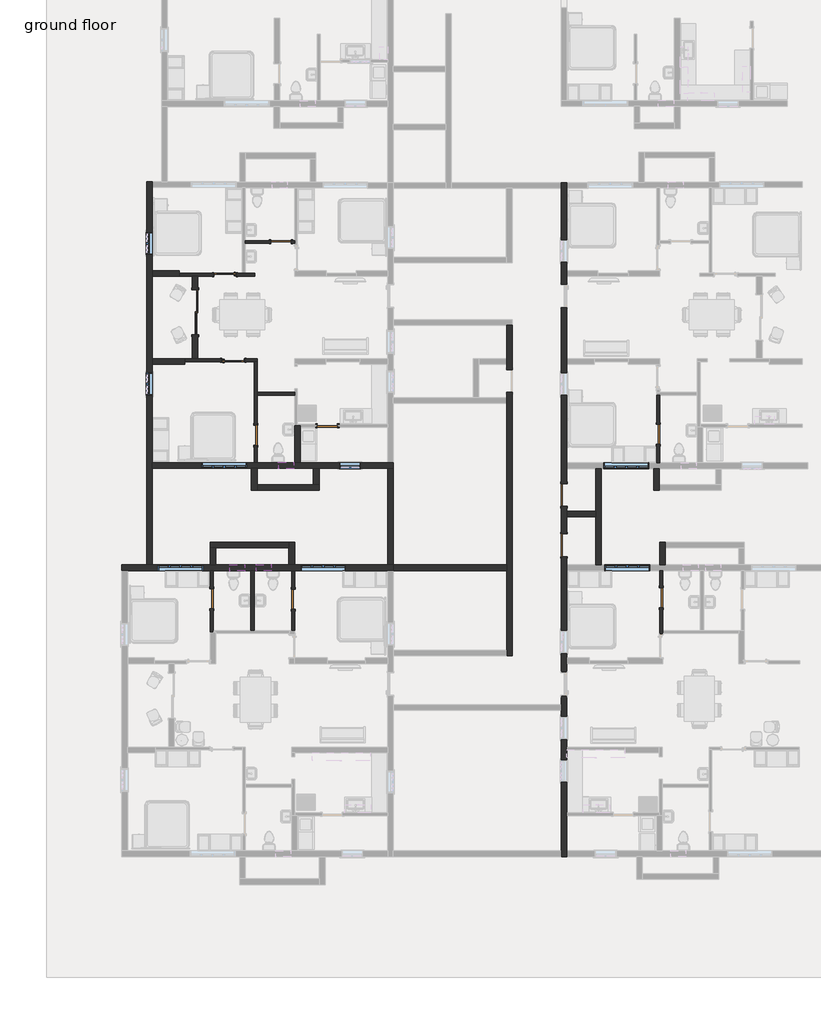
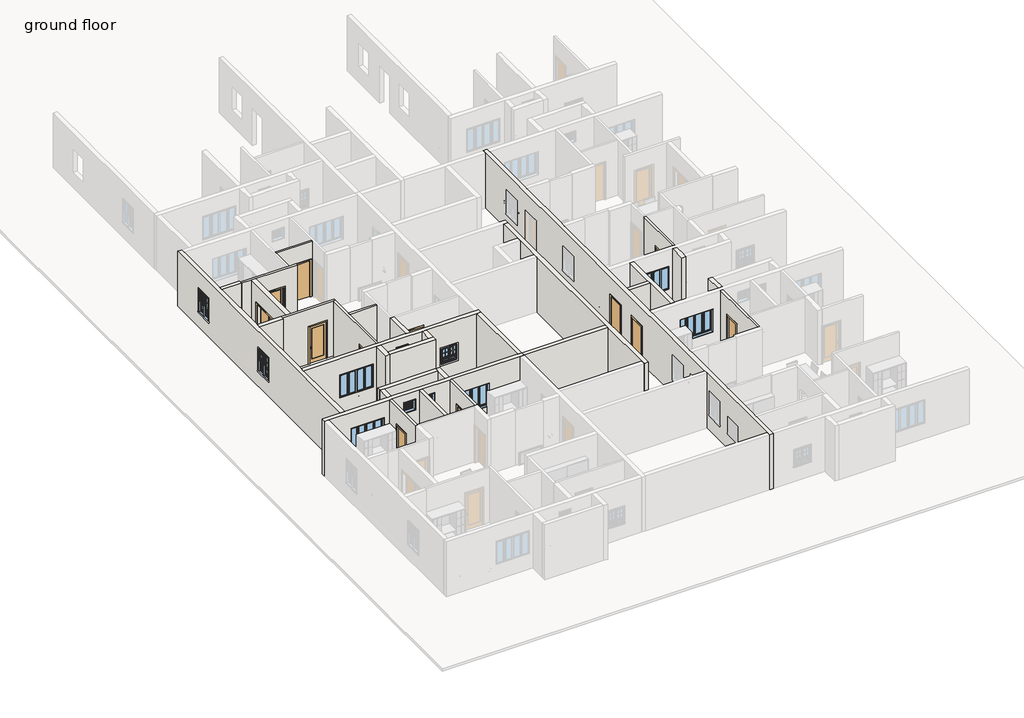
# One storey, part 2 of 16: 31 walls, 12 doors, 11 windows.
"""IFC4 building model written with IfcOpenShell, lengths in millimetres."""

from ifc_helpers import new_model, si_unit, frame, origin, place, context, project, spatial, polyline, outline, extrude, faceted_brep, transform, mapped, element, save
from components import door_d4d75d1e, door_a3feeac7, door_38851409, door_d141acb4, door_0ca8825f, window_ced37e8f, window_5487fb6d, window_f2d8fef0, window_45970670

model = new_model("IFC4")

# Units and contexts
model_context = context("Model", 3, world=origin())
ifc_project = project(units=[si_unit("LENGTHUNIT", "METRE", prefix="MILLI")], contexts=[model_context])

# Site, building, storey
site = spatial("IfcSite", under=ifc_project)
building = spatial("IfcBuilding", under=site)
storey = spatial("IfcBuildingStorey", under=building, Name="ground floor", Elevation=609.6)

# Doors
placement = place(None, origin())
door_shape = door_d4d75d1e(model_context)
element("IfcDoor", 1, ObjectType="Door-Double-Sliding : 72\" x 84\"", at=placement, inside=storey, context=model_context, shape_type="MappedRepresentation", body=[
    mapped(door_shape, transform((44373.526243, -3261.4613664, 609.6), x_axis=(0.0, -1.0, 0.0), y_axis=(1.0, 0.0, 0.0), z_axis=(0.0, 0.0, 1.0))),
])
door_2_shape = door_a3feeac7(model_context)
element("IfcDoor", 2, ObjectType="Door-Interior-Single-1_Panel-Wood : 36\" x 84\"", at=placement, inside=storey, context=model_context, shape_type="MappedRepresentation", body=[
    mapped(door_2_shape, transform((45713.376243, -1734.2863664, 609.6), x_axis=(-1.0, 0.0, 0.0), y_axis=(0.0, -1.0, 0.0), z_axis=(0.0, 0.0, 1.0))),
])
element("IfcDoor", 3, ObjectType="Door-Interior-Single-1_Panel-Wood : 36\" x 84\"", at=placement, inside=storey, context=model_context, shape_type="MappedRepresentation", body=[
    mapped(door_2_shape, transform((46043.576243, -5207.7363664, 609.6), x_axis=(1.0, 0.0, 0.0), y_axis=(0.0, 1.0, 0.0), z_axis=(0.0, 0.0, 1.0))),
])
door_3_shape = door_38851409(model_context)
element("IfcDoor", 4, ObjectType="Single-Flush : 32\" x 84\"", at=placement, inside=storey, context=model_context, shape_type="MappedRepresentation", body=[
    mapped(door_3_shape, transform((63299.8812819, -8216.4424723, 609.6), x_axis=(0.0, 1.0, 0.0), y_axis=(-1.0, 0.0, 0.0), z_axis=(0.0, 0.0, 1.0))),
])
element("IfcDoor", 5, ObjectType="Single-Flush : 32\" x 84\"", at=placement, inside=storey, context=model_context, shape_type="MappedRepresentation", body=[
    mapped(door_3_shape, transform((46957.976243, -8252.8253443, 609.6), x_axis=(0.0, 1.0, 0.0), y_axis=(-1.0, 0.0, 0.0), z_axis=(0.0, 0.0, 1.0))),
])
element("IfcDoor", 6, ObjectType="Single-Flush : 32\" x 84\"", at=placement, inside=storey, context=model_context, shape_type="MappedRepresentation", body=[
    mapped(door_3_shape, transform((47986.676243, -403.9613664, 609.6), x_axis=(-1.0, 0.0, 0.0), y_axis=(0.0, -1.0, 0.0), z_axis=(0.0, 0.0, 1.0))),
])
element("IfcDoor", 7, ObjectType="Single-Flush : 32\" x 84\"", at=placement, inside=storey, context=model_context, shape_type="MappedRepresentation", body=[
    mapped(door_3_shape, transform((48486.1657505, -14903.6865909, 609.6), x_axis=(0.0, -1.0, 0.0), y_axis=(1.0, 0.0, 0.0), z_axis=(0.0, 0.0, 1.0))),
])
door_4_shape = door_d141acb4(model_context)
element("IfcDoor", 8, ObjectType="Single-Flush : 32\" x 84\"", at=placement, inside=storey, context=model_context, shape_type="MappedRepresentation", body=[
    mapped(door_4_shape, transform((49872.626243, -7858.8613664, 609.6), x_axis=(-1.0, 0.0, 0.0), y_axis=(0.0, -1.0, 0.0), z_axis=(0.0, 0.0, 1.0))),
])
element("IfcDoor", 9, ObjectType="Single-Flush : 32\" x 84\"", at=placement, inside=storey, context=model_context, shape_type="MappedRepresentation", body=[
    mapped(door_4_shape, transform((63414.1812819, -14846.5365909, 609.6), x_axis=(0.0, -1.0, 0.0), y_axis=(1.0, 0.0, 0.0), z_axis=(0.0, 0.0, 1.0))),
])
element("IfcDoor", 10, ObjectType="Single-Flush : 32\" x 84\"", at=placement, inside=storey, context=model_context, shape_type="MappedRepresentation", body=[
    mapped(door_4_shape, transform((45170.5764835, -14881.4615909, 609.6), x_axis=(0.0, -1.0, 0.0), y_axis=(1.0, 0.0, 0.0), z_axis=(0.0, 0.0, 1.0))),
])
door_5_shape = door_0ca8825f(model_context)
element("IfcDoor", 11, ObjectType="Single-Flush : 36\" x 84\"", at=placement, inside=storey, context=model_context, shape_type="MappedRepresentation", body=[
    mapped(door_5_shape, transform((59470.8312819, -10676.4239787, 609.6), x_axis=(0.0, 1.0, 0.0), y_axis=(-1.0, 0.0, 0.0), z_axis=(0.0, 0.0, 1.0))),
])
element("IfcDoor", 12, ObjectType="Single-Flush : 36\" x 84\"", at=placement, inside=storey, context=model_context, shape_type="MappedRepresentation", body=[
    mapped(door_5_shape, transform((59470.8312819, -12712.9365909, 609.6), x_axis=(0.0, 1.0, 0.0), y_axis=(-1.0, 0.0, 0.0), z_axis=(0.0, 0.0, 1.0))),
])

# Walls
element("IfcWall", 13, ObjectType="Generic - 4.5\"", at=placement, inside=storey, context=model_context, shape_type="Brep", body=[
    faceted_brep([(43851.5274525, -1680.3113664, 609.6), (43851.5274525, -1680.3113664, 3810.0), (46418.226243, -1680.3113664, 3810.0), (46532.526243, -1680.3113664, 3810.0), (46913.6306279, -1680.3113664, 3810.0), (46913.6306279, -1680.3113664, 609.6), (46532.526243, -1680.3113664, 609.6), (46418.226243, -1680.3113664, 609.6), (46195.976243, -1680.3113664, 609.6), (46195.976243, -1680.3113664, 2768.6), (45230.776243, -1680.3113664, 2768.6), (45230.776243, -1680.3113664, 609.6), (43851.5274525, -1794.6113664, 3810.0), (43851.5274525, -1794.6113664, 609.6), (44386.226243, -1794.6113664, 609.6), (44614.826243, -1794.6113664, 609.6), (45230.776243, -1794.6113664, 609.6), (45230.776243, -1794.6113664, 2768.6), (46195.976243, -1794.6113664, 2768.6), (46195.976243, -1794.6113664, 609.6), (46913.6306279, -1794.6113664, 609.6), (46913.6306279, -1794.6113664, 3810.0), (44614.826243, -1794.6113664, 3810.0), (44386.226243, -1794.6113664, 3810.0)], [[[0, 1, 2, 3, 4, 5, 6, 7, 8, 9, 10, 11]], [[12, 13, 14, 15, 16, 17, 18, 19, 20, 21, 22, 23]], [[5, 20, 19, 8, 7, 6]], [[13, 0, 11, 16, 15, 14]], [[1, 0, 13, 12]], [[4, 3, 2, 1, 12, 23, 22, 21]], [[5, 4, 21, 20]], [[10, 17, 16, 11]], [[17, 10, 9, 18]], [[18, 9, 8, 19]]]),
])
element("IfcWall", 14, ObjectType="Generic - 4.5\"", at=placement, inside=storey, context=model_context, shape_type="SweptSolid", body=[
    extrude(outline(polyline([(609.6, 46532.526243), (609.6, 47580.276243), (2743.2, 47580.276243), (2743.2, 48393.076243), (609.6, 48393.076243), (609.6, 48539.126243), (3810.0, 48539.126243), (3810.0, 46532.526243), (609.6, 46532.526243)])), frame((0.0, -461.1113664, 0.0), z_axis=(0.0, 1.0, 0.0), x_axis=(0.0, 0.0, 1.0)), (0.0, 0.0, 1.0), 114.3),
])
element("IfcWall", 15, ObjectType="Generic - 4.5\"", at=placement, inside=storey, context=model_context, shape_type="Brep", body=[
    faceted_brep([(47015.126243, -5261.7113664, 3810.0), (46900.826243, -5261.7113664, 3810.0), (44081.426243, -5261.7113664, 3810.0), (44081.426243, -5261.7113664, 609.6), (45560.976243, -5261.7113664, 609.6), (45560.976243, -5261.7113664, 2768.6), (46526.176243, -5261.7113664, 2768.6), (46526.176243, -5261.7113664, 609.6), (46900.826243, -5261.7113664, 609.6), (47015.126243, -5261.7113664, 609.6), (44081.426243, -5147.4113664, 3810.0), (44386.226243, -5147.4113664, 3810.0), (44614.826243, -5147.4113664, 3810.0), (47015.126243, -5147.4113664, 3810.0), (47015.126243, -5147.4113664, 609.6), (46526.176243, -5147.4113664, 609.6), (46526.176243, -5147.4113664, 2768.6), (45560.976243, -5147.4113664, 2768.6), (45560.976243, -5147.4113664, 609.6), (44614.826243, -5147.4113664, 609.6), (44386.226243, -5147.4113664, 609.6), (44081.426243, -5147.4113664, 609.6)], [[[0, 1, 2, 3, 4, 5, 6, 7, 8, 9]], [[10, 11, 12, 13, 14, 15, 16, 17, 18, 19, 20, 21]], [[3, 21, 20, 19, 18, 4]], [[14, 9, 8, 7, 15]], [[2, 1, 0, 13, 12, 11, 10]], [[3, 2, 10, 21]], [[0, 9, 14, 13]], [[6, 16, 15, 7]], [[16, 6, 5, 17]], [[17, 5, 4, 18]]]),
])
element("IfcWall", 16, ObjectType="Generic - 4.5\"", at=placement, inside=storey, context=model_context, shape_type="Brep", body=[
    faceted_brep([(46900.826243, -5261.7113664, 609.6), (46900.826243, -7846.4253443, 609.6), (46900.826243, -7846.4253443, 2743.2), (46900.826243, -8659.2253443, 2743.2), (46900.826243, -8659.2253443, 609.6), (46900.826243, -9357.7253443, 609.6), (46900.826243, -9357.7253443, 3810.0), (46900.826243, -5261.7113664, 3810.0), (47015.126243, -7846.4253443, 2743.2), (47015.126243, -7846.4253443, 609.6), (47015.126243, -6620.6113664, 609.6), (47015.126243, -6506.3113664, 609.6), (47015.126243, -5261.7113664, 609.6), (47015.126243, -5261.7113664, 3810.0), (47015.126243, -6506.3113664, 3810.0), (47015.126243, -6620.6113664, 3810.0), (47015.126243, -9357.7253443, 3810.0), (47015.126243, -9357.7253443, 609.6), (47015.126243, -8659.2253443, 609.6), (47015.126243, -8659.2253443, 2743.2)], [[[0, 1, 2, 3, 4, 5, 6, 7]], [[8, 9, 10, 11, 12, 13, 14, 15, 16, 17, 18, 19]], [[18, 17, 5, 4]], [[12, 11, 10, 9, 1, 0]], [[7, 6, 16, 15, 14, 13]], [[0, 7, 13, 12]], [[6, 5, 17, 16]], [[2, 1, 9, 8]], [[3, 2, 8, 19]], [[4, 3, 19, 18]]]),
])
element("IfcWall", 17, ObjectType="Generic - 4.5\"", at=placement, inside=storey, context=model_context, shape_type="SweptSolid", body=[
    extrude(outline(polyline([(48539.126243, -6620.6113664), (47015.126243, -6620.6113664), (47015.126243, -6506.3113664), (48539.126243, -6506.3113664), (48539.126243, -6620.6113664)])), frame((0.0, 0.0, 609.6), z_axis=(0.0, 0.0, 1.0), x_axis=(1.0, 0.0, 0.0)), (0.0, 0.0, 1.0), 3200.4),
])
element("IfcWall", 18, ObjectType="Generic - 4.5\"", at=placement, inside=storey, context=model_context, shape_type="SweptSolid", body=[
    extrude(outline(polyline([(-6620.6113664, 609.6), (-7810.0424723, 609.6), (-7810.0424723, 2743.2), (-8622.8424723, 2743.2), (-8622.8424723, 609.6), (-9372.1424723, 609.6), (-9372.1424723, 3810.0), (-6620.6113664, 3810.0), (-6620.6113664, 609.6)])), frame((63242.7312819, 0.0, 0.0), z_axis=(1.0, 0.0, 0.0), x_axis=(0.0, 1.0, 0.0)), (0.0, 0.0, 1.0), 114.3),
])
element("IfcWall", 19, ObjectType="Generic - 4.5\"", at=placement, inside=storey, context=model_context, shape_type="Brep", body=[
    faceted_brep([(45113.4264835, -15287.8615909, 2743.2), (45113.4264835, -15287.8615909, 609.6), (45113.4264835, -16237.1865909, 609.6), (45113.4264835, -16237.1865909, 3810.0), (45113.4264835, -13741.6365909, 3810.0), (45113.4264835, -13741.6365909, 609.6), (45113.4264835, -14475.0615909, 609.6), (45113.4264835, -14475.0615909, 2743.2), (45227.7264835, -16237.1865909, 609.6), (45227.7264835, -16180.0365909, 609.6), (45227.7264835, -15287.8615909, 609.6), (45227.7264835, -15287.8615909, 2743.2), (45227.7264835, -14475.0615909, 2743.2), (45227.7264835, -14475.0615909, 609.6), (45227.7264835, -13741.6365909, 609.6), (45227.7264835, -13741.6365909, 3810.0), (45227.7264835, -16180.0365909, 3810.0), (45227.7264835, -16237.1865909, 3810.0)], [[[0, 1, 2, 3, 4, 5, 6, 7]], [[8, 9, 10, 11, 12, 13, 14, 15, 16, 17]], [[6, 5, 14, 13]], [[2, 1, 10, 9, 8]], [[3, 2, 8, 17]], [[4, 3, 17, 16, 15]], [[5, 4, 15, 14]], [[11, 10, 1, 0]], [[12, 11, 0, 7]], [[13, 12, 7, 6]]]),
])
element("IfcWall", 20, ObjectType="Generic - 4.5\"", at=placement, inside=storey, context=model_context, shape_type="SweptSolid", body=[
    extrude(outline(polyline([(-15310.0865909, 2743.2), (-15310.0865909, 609.6), (-16180.0365909, 609.6), (-16180.0365909, 3810.0), (-13741.6365909, 3810.0), (-13741.6365909, 609.6), (-14497.2865909, 609.6), (-14497.2865909, 2743.2), (-15310.0865909, 2743.2)])), frame((48429.0157505, 0.0, 0.0), z_axis=(1.0, 0.0, 0.0), x_axis=(0.0, 1.0, 0.0)), (0.0, 0.0, 1.0), 114.3),
])
element("IfcWall", 21, ObjectType="Generic - 4.5\"", at=placement, inside=storey, context=model_context, shape_type="Brep", body=[
    faceted_brep([(63357.0312819, -15252.9365909, 2743.2), (63357.0312819, -15252.9365909, 609.6), (63357.0312819, -16335.6115909, 609.6), (63357.0312819, -16335.6115909, 2768.6), (63357.0312819, -17284.9365909, 2768.6), (63357.0312819, -17284.9365909, 3810.0), (63357.0312819, -13741.6365909, 3810.0), (63357.0312819, -13741.6365909, 609.6), (63357.0312819, -14440.1365909, 609.6), (63357.0312819, -14440.1365909, 2743.2), (63471.3312819, -16335.6115909, 609.6), (63471.3312819, -16294.3365909, 609.6), (63471.3312819, -16180.0365909, 609.6), (63471.3312819, -15252.9365909, 609.6), (63471.3312819, -15252.9365909, 2743.2), (63471.3312819, -14440.1365909, 2743.2), (63471.3312819, -14440.1365909, 609.6), (63471.3312819, -13741.6365909, 609.6), (63471.3312819, -13741.6365909, 3810.0), (63471.3312819, -16180.0365909, 3810.0), (63471.3312819, -16294.3365909, 3810.0), (63471.3312819, -17284.9365909, 3810.0), (63471.3312819, -17284.9365909, 2768.6), (63471.3312819, -16335.6115909, 2768.6)], [[[0, 1, 2, 3, 4, 5, 6, 7, 8, 9]], [[10, 11, 12, 13, 14, 15, 16, 17, 18, 19, 20, 21, 22, 23]], [[8, 7, 17, 16]], [[2, 1, 13, 12, 11, 10]], [[6, 5, 21, 20, 19, 18]], [[21, 5, 4, 22]], [[7, 6, 18, 17]], [[3, 23, 22, 4]], [[23, 3, 2, 10]], [[14, 13, 1, 0]], [[15, 14, 0, 9]], [[16, 15, 9, 8]]]),
])
element("IfcWall", 22, ObjectType="Generic - 6\"", at=placement, inside=storey, context=model_context, shape_type="SweptSolid", body=[
    extrude(outline(polyline([(46748.426243, -16180.0365909), (46748.426243, -13741.6365909), (46900.826243, -13741.6365909), (46900.826243, -16180.0365909), (46748.426243, -16180.0365909)])), frame((0.0, 0.0, 609.6), z_axis=(0.0, 0.0, 1.0), x_axis=(1.0, 0.0, 0.0)), (0.0, 0.0, 1.0), 3200.4),
])
element("IfcWall", 23, ObjectType="Generic - 9\"", at=placement, inside=storey, context=model_context, shape_type="Brep", body=[
    faceted_brep([(42532.026243, 2046.8746557, 609.6), (42532.026243, -13513.0365909, 609.6), (42532.026243, -13513.0365909, 3810.0), (42532.026243, 2046.8746557, 3810.0), (42532.026243, -6633.3113664, 2844.8), (42532.026243, -6633.3113664, 1524.0), (42532.026243, -5718.9113664, 1524.0), (42532.026243, -5718.9113664, 2844.8), (42532.026243, -918.3113664, 2844.8), (42532.026243, -918.3113664, 1524.0), (42532.026243, -3.9113664, 1524.0), (42532.026243, -3.9113664, 2844.8), (42760.626243, 2045.9651274, 609.6), (42760.626243, 2045.9651274, 3810.0), (42760.626243, 1817.363318, 3810.0), (42760.626243, -1566.0113664, 3810.0), (42760.626243, -1794.6113664, 3810.0), (42760.626243, -5147.4113664, 3810.0), (42760.626243, -5376.0113664, 3810.0), (42760.626243, -9357.7253443, 3810.0), (42760.626243, -9586.3253443, 3810.0), (42760.626243, -13513.0365909, 3810.0), (42760.626243, -13513.0365909, 609.6), (42760.626243, -9586.3253443, 609.6), (42760.626243, -9357.7253443, 609.6), (42760.626243, -5376.0113664, 609.6), (42760.626243, -5147.4113664, 609.6), (42760.626243, -1794.6113664, 609.6), (42760.626243, -1566.0113664, 609.6), (42760.626243, 1817.363318, 609.6), (42760.626243, -6633.3113664, 2844.8), (42760.626243, -5718.9113664, 2844.8), (42760.626243, -5718.9113664, 1524.0), (42760.626243, -6633.3113664, 1524.0), (42760.626243, -918.3113664, 2844.8), (42760.626243, -3.9113664, 2844.8), (42760.626243, -3.9113664, 1524.0), (42760.626243, -918.3113664, 1524.0)], [[[0, 1, 2, 3], [4, 5, 6, 7], [8, 9, 10, 11]], [[12, 13, 14, 15, 16, 17, 18, 19, 20, 21, 22, 23, 24, 25, 26, 27, 28, 29], [30, 31, 32, 33], [34, 35, 36, 37]], [[1, 0, 12, 29, 28, 27, 26, 25, 24, 23, 22]], [[3, 2, 21, 20, 19, 18, 17, 16, 15, 14, 13]], [[0, 3, 13, 12]], [[2, 1, 22, 21]], [[5, 4, 30, 33]], [[6, 5, 33, 32]], [[7, 6, 32, 31]], [[4, 7, 31, 30]], [[9, 8, 34, 37]], [[10, 9, 37, 36]], [[11, 10, 36, 35]], [[8, 11, 35, 34]]]),
])
element("IfcWall", 24, ObjectType="Generic - 9\"", at=placement, inside=storey, context=model_context, shape_type="Brep", body=[
    faceted_brep([(42760.626243, -9586.3253443, 609.6), (46786.526243, -9586.3253443, 609.6), (47015.126243, -9586.3253443, 609.6), (49300.2509253, -9586.3253443, 609.6), (49528.8509253, -9586.3253443, 609.6), (52311.026243, -9586.3253443, 609.6), (52539.626243, -9586.3253443, 609.6), (52539.626243, -9586.3253443, 3810.0), (52311.026243, -9586.3253443, 3810.0), (49528.8509253, -9586.3253443, 3810.0), (49300.2509253, -9586.3253443, 3810.0), (47015.126243, -9586.3253443, 3810.0), (46786.526243, -9586.3253443, 3810.0), (42760.626243, -9586.3253443, 3810.0), (44767.226243, -9586.3253443, 2870.2), (46596.026243, -9586.3253443, 2870.2), (46596.026243, -9586.3253443, 1524.0), (44767.226243, -9586.3253443, 1524.0), (50354.3509253, -9586.3253443, 2438.4), (51217.9509253, -9586.3253443, 2438.4), (51217.9509253, -9586.3253443, 1524.0), (50354.3509253, -9586.3253443, 1524.0), (48501.026243, -9586.3253443, 3352.8), (48501.026243, -9586.3253443, 2743.2), (47891.426243, -9586.3253443, 2743.2), (47891.426243, -9586.3253443, 3352.8), (42760.626243, -9357.7253443, 609.6), (42760.626243, -9357.7253443, 3810.0), (46900.826243, -9357.7253443, 3810.0), (47015.126243, -9357.7253443, 3810.0), (48539.126243, -9357.7253443, 3810.0), (48767.726243, -9357.7253443, 3810.0), (52311.026243, -9357.7253443, 3810.0), (52539.626243, -9357.7253443, 3810.0), (52539.626243, -9357.7253443, 609.6), (52311.026243, -9357.7253443, 609.6), (48767.726243, -9357.7253443, 609.6), (48539.126243, -9357.7253443, 609.6), (47015.126243, -9357.7253443, 609.6), (46900.826243, -9357.7253443, 609.6), (44767.226243, -9357.7253443, 2870.2), (44767.226243, -9357.7253443, 1524.0), (46596.026243, -9357.7253443, 1524.0), (46596.026243, -9357.7253443, 2870.2), (50354.3509253, -9357.7253443, 2438.4), (50354.3509253, -9357.7253443, 1524.0), (51217.9509253, -9357.7253443, 1524.0), (51217.9509253, -9357.7253443, 2438.4), (48501.026243, -9357.7253443, 3352.8), (47891.426243, -9357.7253443, 3352.8), (47891.426243, -9357.7253443, 2743.2), (48501.026243, -9357.7253443, 2743.2)], [[[0, 1, 2, 3, 4, 5, 6, 7, 8, 9, 10, 11, 12, 13], [14, 15, 16, 17], [18, 19, 20, 21], [22, 23, 24, 25]], [[26, 27, 28, 29, 30, 31, 32, 33, 34, 35, 36, 37, 38, 39], [40, 41, 42, 43], [44, 45, 46, 47], [48, 49, 50, 51]], [[6, 5, 4, 3, 2, 1, 0, 26, 39, 38, 37, 36, 35, 34]], [[13, 12, 11, 10, 9, 8, 7, 33, 32, 31, 30, 29, 28, 27]], [[0, 13, 27, 26]], [[7, 6, 34, 33]], [[41, 40, 14, 17]], [[42, 41, 17, 16]], [[43, 42, 16, 15]], [[40, 43, 15, 14]], [[45, 44, 18, 21]], [[46, 45, 21, 20]], [[47, 46, 20, 19]], [[44, 47, 19, 18]], [[23, 22, 48, 51]], [[24, 23, 51, 50]], [[25, 24, 50, 49]], [[22, 25, 49, 48]]]),
])
element("IfcWall", 25, ObjectType="Generic - 9\"", at=placement, inside=storey, context=model_context, shape_type="Brep", body=[
    faceted_brep([(42760.626243, -1794.6113664, 609.6), (43851.5274525, -1794.6113664, 609.6), (43851.5274525, -1794.6113664, 3810.0), (42760.626243, -1794.6113664, 3810.0), (42760.626243, -1566.0113664, 609.6), (42760.626243, -1566.0113664, 3810.0), (43851.5274525, -1566.0113664, 3810.0), (43851.5274525, -1566.0113664, 609.6), (43851.5274525, -1680.3113664, 609.6), (43851.5274525, -1680.3113664, 3810.0)], [[[0, 1, 2, 3]], [[4, 5, 6, 7]], [[1, 0, 4, 7, 8]], [[2, 1, 8, 7, 6, 9]], [[3, 2, 9, 6, 5]], [[0, 3, 5, 4]]]),
])
element("IfcWall", 26, ObjectType="Generic - 9\"", at=placement, inside=storey, context=model_context, shape_type="SweptSolid", body=[
    extrude(outline(polyline([(-4175.8613664, 2743.2), (-4175.8613664, 609.6), (-5147.4113664, 609.6), (-5147.4113664, 3810.0), (-1794.6113664, 3810.0), (-1794.6113664, 609.6), (-2347.0613664, 609.6), (-2347.0613664, 2743.2), (-4175.8613664, 2743.2)])), frame((44386.226243, 0.0, 0.0), z_axis=(1.0, 0.0, 0.0), x_axis=(0.0, 1.0, 0.0)), (0.0, 0.0, 1.0), 228.6),
])
element("IfcWall", 27, ObjectType="Generic - 9\"", at=placement, inside=storey, context=model_context, shape_type="Brep", body=[
    faceted_brep([(42760.626243, -5376.0113664, 609.6), (44081.426243, -5376.0113664, 609.6), (44081.426243, -5376.0113664, 3810.0), (42760.626243, -5376.0113664, 3810.0), (42760.626243, -5147.4113664, 609.6), (42760.626243, -5147.4113664, 3810.0), (44081.426243, -5147.4113664, 3810.0), (44081.426243, -5147.4113664, 609.6), (44081.426243, -5261.7113664, 609.6), (44081.426243, -5261.7113664, 3810.0)], [[[0, 1, 2, 3]], [[4, 5, 6, 7]], [[1, 0, 4, 7, 8]], [[2, 1, 8, 7, 6, 9]], [[3, 2, 9, 6, 5]], [[0, 3, 5, 4]]]),
])
element("IfcWall", 28, ObjectType="Generic - 9\"", at=placement, inside=storey, context=model_context, shape_type="Brep", body=[
    faceted_brep([(48767.726243, -9357.7253443, 609.6), (48767.726243, -7916.0113664, 609.6), (48767.726243, -7858.8613664, 609.6), (48767.726243, -7858.8613664, 3810.0), (48767.726243, -7916.0113664, 3810.0), (48767.726243, -9357.7253443, 3810.0), (48539.126243, -9357.7253443, 609.6), (48539.126243, -9357.7253443, 3810.0), (48539.126243, -7858.8613664, 3810.0), (48539.126243, -7858.8613664, 609.6), (48653.426243, -7858.8613664, 609.6), (48653.426243, -7858.8613664, 3810.0)], [[[0, 1, 2, 3, 4, 5]], [[6, 7, 8, 9]], [[2, 1, 0, 6, 9, 10]], [[3, 2, 10, 9, 8, 11]], [[5, 4, 3, 11, 8, 7]], [[0, 5, 7, 6]]]),
])
element("IfcWall", 29, ObjectType="Generic - 9\"", at=placement, inside=storey, context=model_context, shape_type="Brep", body=[
    faceted_brep([(63108.7268416, -9600.7424723, 609.6), (63108.7268416, -10476.6021216, 609.6), (63108.7268416, -10476.6021216, 3810.0), (63108.7268416, -9600.7424723, 3810.0), (63337.3268416, -9600.7424723, 609.6), (63337.3268416, -9600.7424723, 3810.0), (63337.3268416, -10248.0021216, 3810.0), (63337.3268416, -10476.6021216, 3810.0), (63337.3268416, -10476.6021216, 609.6), (63337.3268416, -10248.0021216, 609.6)], [[[0, 1, 2, 3]], [[4, 5, 6, 7, 8, 9]], [[1, 0, 4, 9, 8]], [[3, 2, 7, 6, 5]], [[0, 3, 5, 4]], [[2, 1, 8, 7]]]),
])
element("IfcWall", 30, ObjectType="Generic - 9\"", at=placement, inside=storey, context=model_context, shape_type="Brep", body=[
    faceted_brep([(46786.526243, -9586.3253443, 609.6), (46786.526243, -10476.6021216, 609.6), (46786.526243, -10476.6021216, 3810.0), (46786.526243, -9586.3253443, 3810.0), (47015.126243, -9586.3253443, 609.6), (47015.126243, -9586.3253443, 3810.0), (47015.126243, -10248.0021216, 3810.0), (47015.126243, -10476.6021216, 3810.0), (47015.126243, -10476.6021216, 609.6), (47015.126243, -10248.0021216, 609.6)], [[[0, 1, 2, 3]], [[4, 5, 6, 7, 8, 9]], [[1, 0, 4, 9, 8]], [[3, 2, 7, 6, 5]], [[0, 3, 5, 4]], [[2, 1, 8, 7]]]),
])
element("IfcWall", 31, ObjectType="Generic - 9\"", at=placement, inside=storey, context=model_context, shape_type="Brep", body=[
    faceted_brep([(47015.126243, -10476.6021216, 609.6), (49528.8509253, -10476.6021216, 609.6), (49528.8509253, -10476.6021216, 3810.0), (47015.126243, -10476.6021216, 3810.0), (47015.126243, -10248.0021216, 609.6), (47015.126243, -10248.0021216, 3810.0), (49300.2509253, -10248.0021216, 3810.0), (49528.8509253, -10248.0021216, 3810.0), (49528.8509253, -10248.0021216, 609.6), (49300.2509253, -10248.0021216, 609.6)], [[[0, 1, 2, 3]], [[4, 5, 6, 7, 8, 9]], [[1, 0, 4, 9, 8]], [[3, 2, 7, 6, 5]], [[0, 3, 5, 4]], [[2, 1, 8, 7]]]),
])
element("IfcWall", 32, ObjectType="Generic - 9\"", at=placement, inside=storey, context=model_context, shape_type="SweptSolid", body=[
    extrude(outline(polyline([(49528.8509253, -9586.3253443), (49528.8509253, -10248.0021216), (49300.2509253, -10248.0021216), (49300.2509253, -9586.3253443), (49528.8509253, -9586.3253443)])), frame((0.0, 0.0, 609.6), z_axis=(0.0, 0.0, 1.0), x_axis=(1.0, 0.0, 0.0)), (0.0, 0.0, 1.0), 3200.4),
])
element("IfcWall", 33, ObjectType="Generic - 9\"", at=placement, inside=storey, context=model_context, shape_type="Brep", body=[
    faceted_brep([(41528.726243, -13741.6365909, 609.6), (41757.326243, -13741.6365909, 609.6), (45113.4264835, -13741.6365909, 609.6), (45227.7264835, -13741.6365909, 609.6), (46748.426243, -13741.6365909, 609.6), (46900.826243, -13741.6365909, 609.6), (48429.0157505, -13741.6365909, 609.6), (48543.3157505, -13741.6365909, 609.6), (52311.026243, -13741.6365909, 609.6), (52539.626243, -13741.6365909, 609.6), (52539.626243, -13741.6365909, 3810.0), (52311.026243, -13741.6365909, 3810.0), (48543.3157505, -13741.6365909, 3810.0), (48429.0157505, -13741.6365909, 3810.0), (46900.826243, -13741.6365909, 3810.0), (46748.426243, -13741.6365909, 3810.0), (45227.7264835, -13741.6365909, 3810.0), (45113.4264835, -13741.6365909, 3810.0), (41757.326243, -13741.6365909, 3810.0), (41528.726243, -13741.6365909, 3810.0), (44822.8513633, -13741.6365909, 2870.2), (44822.8513633, -13741.6365909, 1524.0), (42994.0513633, -13741.6365909, 1524.0), (42994.0513633, -13741.6365909, 2870.2), (50619.7657505, -13741.6365909, 2870.2), (50619.7657505, -13741.6365909, 1524.0), (48790.9657505, -13741.6365909, 1524.0), (48790.9657505, -13741.6365909, 2870.2), (46977.026243, -13741.6365909, 3352.8), (47586.626243, -13741.6365909, 3352.8), (47586.626243, -13741.6365909, 2743.2), (46977.026243, -13741.6365909, 2743.2), (45910.226243, -13741.6365909, 3352.8), (46519.826243, -13741.6365909, 3352.8), (46519.826243, -13741.6365909, 2743.2), (45910.226243, -13741.6365909, 2743.2), (41528.726243, -13513.0365909, 609.6), (41528.726243, -13513.0365909, 3810.0), (42532.026243, -13513.0365909, 3810.0), (42760.626243, -13513.0365909, 3810.0), (45113.4264835, -13513.0365909, 3810.0), (45342.0264835, -13513.0365909, 3810.0), (48310.526243, -13513.0365909, 3810.0), (48539.126243, -13513.0365909, 3810.0), (52311.026243, -13513.0365909, 3810.0), (52539.626243, -13513.0365909, 3810.0), (52539.626243, -13513.0365909, 609.6), (52311.026243, -13513.0365909, 609.6), (48539.126243, -13513.0365909, 609.6), (48310.526243, -13513.0365909, 609.6), (45342.0264835, -13513.0365909, 609.6), (45113.4264835, -13513.0365909, 609.6), (42760.626243, -13513.0365909, 609.6), (42532.026243, -13513.0365909, 609.6), (44822.8513633, -13513.0365909, 2870.2), (42994.0513633, -13513.0365909, 2870.2), (42994.0513633, -13513.0365909, 1524.0), (44822.8513633, -13513.0365909, 1524.0), (50619.7657505, -13513.0365909, 2870.2), (48790.9657505, -13513.0365909, 2870.2), (48790.9657505, -13513.0365909, 1524.0), (50619.7657505, -13513.0365909, 1524.0), (46977.026243, -13513.0365909, 3352.8), (46977.026243, -13513.0365909, 2743.2), (47586.626243, -13513.0365909, 2743.2), (47586.626243, -13513.0365909, 3352.8), (45910.226243, -13513.0365909, 3352.8), (45910.226243, -13513.0365909, 2743.2), (46519.826243, -13513.0365909, 2743.2), (46519.826243, -13513.0365909, 3352.8)], [[[0, 1, 2, 3, 4, 5, 6, 7, 8, 9, 10, 11, 12, 13, 14, 15, 16, 17, 18, 19], [20, 21, 22, 23], [24, 25, 26, 27], [28, 29, 30, 31], [32, 33, 34, 35]], [[36, 37, 38, 39, 40, 41, 42, 43, 44, 45, 46, 47, 48, 49, 50, 51, 52, 53], [54, 55, 56, 57], [58, 59, 60, 61], [62, 63, 64, 65], [66, 67, 68, 69]], [[9, 8, 7, 6, 5, 4, 3, 2, 1, 0, 36, 53, 52, 51, 50, 49, 48, 47, 46]], [[19, 18, 17, 16, 15, 14, 13, 12, 11, 10, 45, 44, 43, 42, 41, 40, 39, 38, 37]], [[10, 9, 46, 45]], [[0, 19, 37, 36]], [[21, 20, 54, 57]], [[22, 21, 57, 56]], [[23, 22, 56, 55]], [[20, 23, 55, 54]], [[25, 24, 58, 61]], [[26, 25, 61, 60]], [[27, 26, 60, 59]], [[24, 27, 59, 58]], [[63, 62, 28, 31]], [[64, 63, 31, 30]], [[65, 64, 30, 29]], [[62, 65, 29, 28]], [[67, 66, 32, 35]], [[68, 67, 35, 34]], [[69, 68, 34, 33]], [[66, 69, 33, 32]]]),
])
element("IfcWall", 34, ObjectType="Generic - 9\"", at=placement, inside=storey, context=model_context, shape_type="Brep", body=[
    faceted_brep([(48539.126243, -13513.0365909, 609.6), (48539.126243, -12589.9206064, 609.6), (48539.126243, -12589.9206064, 3810.0), (48539.126243, -13513.0365909, 3810.0), (48310.526243, -13513.0365909, 609.6), (48310.526243, -13513.0365909, 3810.0), (48310.526243, -12818.5206064, 3810.0), (48310.526243, -12589.9206064, 3810.0), (48310.526243, -12589.9206064, 609.6), (48310.526243, -12818.5206064, 609.6)], [[[0, 1, 2, 3]], [[4, 5, 6, 7, 8, 9]], [[1, 0, 4, 9, 8]], [[3, 2, 7, 6, 5]], [[0, 3, 5, 4]], [[2, 1, 8, 7]]]),
])
element("IfcWall", 35, ObjectType="Generic - 9\"", at=placement, inside=storey, context=model_context, shape_type="Brep", body=[
    faceted_brep([(48310.526243, -12589.9206064, 609.6), (45113.4264835, -12589.9206064, 609.6), (45113.4264835, -12589.9206064, 3810.0), (48310.526243, -12589.9206064, 3810.0), (48310.526243, -12818.5206064, 609.6), (48310.526243, -12818.5206064, 3810.0), (45342.0264835, -12818.5206064, 3810.0), (45113.4264835, -12818.5206064, 3810.0), (45113.4264835, -12818.5206064, 609.6), (45342.0264835, -12818.5206064, 609.6)], [[[0, 1, 2, 3]], [[4, 5, 6, 7, 8, 9]], [[1, 0, 4, 9, 8]], [[3, 2, 7, 6, 5]], [[0, 3, 5, 4]], [[2, 1, 8, 7]]]),
])
element("IfcWall", 36, ObjectType="Generic - 9\"", at=placement, inside=storey, context=model_context, shape_type="SweptSolid", body=[
    extrude(outline(polyline([(45113.4264835, -13513.0365909), (45113.4264835, -12818.5206064), (45342.0264835, -12818.5206064), (45342.0264835, -13513.0365909), (45113.4264835, -13513.0365909)])), frame((0.0, 0.0, 609.6), z_axis=(0.0, 0.0, 1.0), x_axis=(1.0, 0.0, 0.0)), (0.0, 0.0, 1.0), 3200.4),
])
element("IfcWall", 37, ObjectType="Generic - 9\"", at=placement, inside=storey, context=model_context, shape_type="Brep", body=[
    faceted_brep([(59356.5312819, -11133.6239787, 609.6), (59356.5312819, -12255.7365909, 609.6), (59356.5312819, -12255.7365909, 2743.2), (59356.5312819, -13170.1365909, 2743.2), (59356.5312819, -13170.1365909, 609.6), (59356.5312819, -17863.851256, 609.6), (59356.5312819, -17863.851256, 2768.6), (59356.5312819, -18829.051256, 2768.6), (59356.5312819, -18829.051256, 609.6), (59356.5312819, -19179.3659211, 609.6), (59356.5312819, -19407.9659211, 609.6), (59356.5312819, -25120.8365909, 609.6), (59356.5312819, -25349.4365909, 609.6), (59356.5312819, -25349.4365909, 3810.0), (59356.5312819, -25120.8365909, 3810.0), (59356.5312819, -19407.9659211, 3810.0), (59356.5312819, -19179.3659211, 3810.0), (59356.5312819, 1769.0590685, 3810.0), (59356.5312819, 1997.6590685, 3810.0), (59356.5312819, 2007.0575277, 3810.0), (59356.5312819, 2007.0575277, 609.6), (59356.5312819, 1997.6590685, 609.6), (59356.5312819, 1769.0590685, 609.6), (59356.5312819, -2112.1113664, 609.6), (59356.5312819, -2112.1113664, 2768.6), (59356.5312819, -3077.3113664, 2768.6), (59356.5312819, -3077.3113664, 609.6), (59356.5312819, -10219.2239787, 609.6), (59356.5312819, -10219.2239787, 2743.2), (59356.5312819, -11133.6239787, 2743.2), (59356.5312819, -17094.4365909, 2844.8), (59356.5312819, -17094.4365909, 1524.0), (59356.5312819, -16180.0365909, 1524.0), (59356.5312819, -16180.0365909, 2844.8), (59356.5312819, -21444.0658586, 2438.4), (59356.5312819, -22307.6658586, 2438.4), (59356.5312819, -22307.6658586, 1524.0), (59356.5312819, -21444.0658586, 1524.0), (59356.5312819, -20584.7658899, 2844.8), (59356.5312819, -20584.7658899, 1524.0), (59356.5312819, -19670.3658899, 1524.0), (59356.5312819, -19670.3658899, 2844.8), (59356.5312819, -6633.3113664, 2844.8), (59356.5312819, -6633.3113664, 1524.0), (59356.5312819, -5718.9113664, 1524.0), (59356.5312819, -5718.9113664, 2844.8), (59356.5312819, -1223.1113664, 2844.8), (59356.5312819, -1223.1113664, 1524.0), (59356.5312819, -308.7113664, 1524.0), (59356.5312819, -308.7113664, 2844.8), (59585.1312819, -12255.7365909, 2743.2), (59585.1312819, -12255.7365909, 609.6), (59585.1312819, -11552.7239787, 609.6), (59585.1312819, -11324.1239787, 609.6), (59585.1312819, -11133.6239787, 609.6), (59585.1312819, -11133.6239787, 2743.2), (59585.1312819, -10219.2239787, 2743.2), (59585.1312819, -10219.2239787, 609.6), (59585.1312819, -9600.7424723, 609.6), (59585.1312819, -9372.1424723, 609.6), (59585.1312819, -5376.0113664, 609.6), (59585.1312819, -5147.4113664, 609.6), (59585.1312819, -3077.3113664, 609.6), (59585.1312819, -3077.3113664, 2768.6), (59585.1312819, -2112.1113664, 2768.6), (59585.1312819, -2112.1113664, 609.6), (59585.1312819, -1794.6113664, 609.6), (59585.1312819, -1566.0113664, 609.6), (59585.1312819, 1779.3652466, 609.6), (59585.1312819, 2007.967056, 609.6), (59585.1312819, 2007.967056, 3810.0), (59585.1312819, 1779.3652466, 3810.0), (59585.1312819, -1566.0113664, 3810.0), (59585.1312819, -1794.6113664, 3810.0), (59585.1312819, -5147.4113664, 3810.0), (59585.1312819, -5376.0113664, 3810.0), (59585.1312819, -9372.1424723, 3810.0), (59585.1312819, -9600.7424723, 3810.0), (59585.1312819, -11324.1239787, 3810.0), (59585.1312819, -11552.7239787, 3810.0), (59585.1312819, -13513.0365909, 3810.0), (59585.1312819, -13741.6365909, 3810.0), (59585.1312819, -17284.9365909, 3810.0), (59585.1312819, -17513.5365909, 3810.0), (59585.1312819, -20904.3158586, 3810.0), (59585.1312819, -21018.6158586, 3810.0), (59585.1312819, -23571.3158586, 3810.0), (59585.1312819, -23685.6158586, 3810.0), (59585.1312819, -25120.8365909, 3810.0), (59585.1312819, -25349.4365909, 3810.0), (59585.1312819, -25349.4365909, 609.6), (59585.1312819, -25120.8365909, 609.6), (59585.1312819, -23685.6158586, 609.6), (59585.1312819, -23571.3158586, 609.6), (59585.1312819, -21018.6158586, 609.6), (59585.1312819, -20904.3158586, 609.6), (59585.1312819, -18829.051256, 609.6), (59585.1312819, -18829.051256, 2768.6), (59585.1312819, -17863.851256, 2768.6), (59585.1312819, -17863.851256, 609.6), (59585.1312819, -17513.5365909, 609.6), (59585.1312819, -17284.9365909, 609.6), (59585.1312819, -13741.6365909, 609.6), (59585.1312819, -13513.0365909, 609.6), (59585.1312819, -13170.1365909, 609.6), (59585.1312819, -13170.1365909, 2743.2), (59585.1312819, -17094.4365909, 2844.8), (59585.1312819, -16180.0365909, 2844.8), (59585.1312819, -16180.0365909, 1524.0), (59585.1312819, -17094.4365909, 1524.0), (59585.1312819, -21444.0658586, 2438.4), (59585.1312819, -21444.0658586, 1524.0), (59585.1312819, -22307.6658586, 1524.0), (59585.1312819, -22307.6658586, 2438.4), (59585.1312819, -20584.7658899, 2844.8), (59585.1312819, -19670.3658899, 2844.8), (59585.1312819, -19670.3658899, 1524.0), (59585.1312819, -20584.7658899, 1524.0), (59585.1312819, -6633.3113664, 2844.8), (59585.1312819, -5718.9113664, 2844.8), (59585.1312819, -5718.9113664, 1524.0), (59585.1312819, -6633.3113664, 1524.0), (59585.1312819, -1223.1113664, 2844.8), (59585.1312819, -308.7113664, 2844.8), (59585.1312819, -308.7113664, 1524.0), (59585.1312819, -1223.1113664, 1524.0)], [[[0, 1, 2, 3, 4, 5, 6, 7, 8, 9, 10, 11, 12, 13, 14, 15, 16, 17, 18, 19, 20, 21, 22, 23, 24, 25, 26, 27, 28, 29], [30, 31, 32, 33], [34, 35, 36, 37], [38, 39, 40, 41], [42, 43, 44, 45], [46, 47, 48, 49]], [[50, 51, 52, 53, 54, 55, 56, 57, 58, 59, 60, 61, 62, 63, 64, 65, 66, 67, 68, 69, 70, 71, 72, 73, 74, 75, 76, 77, 78, 79, 80, 81, 82, 83, 84, 85, 86, 87, 88, 89, 90, 91, 92, 93, 94, 95, 96, 97, 98, 99, 100, 101, 102, 103, 104, 105], [106, 107, 108, 109], [110, 111, 112, 113], [114, 115, 116, 117], [118, 119, 120, 121], [122, 123, 124, 125]], [[90, 12, 11, 10, 9, 8, 96, 95, 94, 93, 92, 91]], [[20, 69, 68, 67, 66, 65, 23, 22, 21]], [[62, 61, 60, 59, 58, 57, 27, 26]], [[104, 103, 102, 101, 100, 99, 5, 4]], [[54, 53, 52, 51, 1, 0]], [[19, 18, 17, 16, 15, 14, 13, 89, 88, 87, 86, 85, 84, 83, 82, 81, 80, 79, 78, 77, 76, 75, 74, 73, 72, 71, 70]], [[13, 12, 90, 89]], [[7, 97, 96, 8]], [[97, 7, 6, 98]], [[98, 6, 5, 99]], [[31, 30, 106, 109]], [[32, 31, 109, 108]], [[33, 32, 108, 107]], [[30, 33, 107, 106]], [[111, 110, 34, 37]], [[112, 111, 37, 36]], [[113, 112, 36, 35]], [[110, 113, 35, 34]], [[39, 38, 114, 117]], [[40, 39, 117, 116]], [[41, 40, 116, 115]], [[38, 41, 115, 114]], [[42, 45, 119, 118]], [[45, 44, 120, 119]], [[44, 43, 121, 120]], [[43, 42, 118, 121]], [[46, 49, 123, 122]], [[49, 48, 124, 123]], [[48, 47, 125, 124]], [[47, 46, 122, 125]], [[20, 19, 70, 69]], [[64, 24, 23, 65]], [[24, 64, 63, 25]], [[25, 63, 62, 26]], [[28, 27, 57, 56]], [[29, 28, 56, 55]], [[0, 29, 55, 54]], [[2, 1, 51, 50]], [[3, 2, 50, 105]], [[4, 3, 105, 104]]]),
])
element("IfcWall", 38, ObjectType="Generic - 9\"", at=placement, inside=storey, context=model_context, shape_type="Brep", body=[
    faceted_brep([(63585.6312819, -13513.0365909, 609.6), (63585.6312819, -12818.5206064, 609.6), (63585.6312819, -12589.9206064, 609.6), (63585.6312819, -12589.9206064, 3810.0), (63585.6312819, -12818.5206064, 3810.0), (63585.6312819, -13513.0365909, 3810.0), (63357.0312819, -13513.0365909, 609.6), (63357.0312819, -13513.0365909, 3810.0), (63357.0312819, -12589.9206064, 3810.0), (63357.0312819, -12589.9206064, 609.6)], [[[0, 1, 2, 3, 4, 5]], [[6, 7, 8, 9]], [[2, 1, 0, 6, 9]], [[5, 4, 3, 8, 7]], [[0, 5, 7, 6]], [[3, 2, 9, 8]]]),
])
element("IfcWall", 39, ObjectType="Generic - 9\"", at=placement, inside=storey, context=model_context, shape_type="Brep", body=[
    faceted_brep([(57146.7312819, -6509.6343195, 2743.2), (57146.7312819, -6509.6343195, 609.6), (57146.7312819, -6728.8572725, 609.6), (57146.7312819, -6957.4572725, 609.6), (57146.7312819, -13513.0365909, 609.6), (57146.7312819, -13741.6365909, 609.6), (57146.7312819, -16969.5659211, 609.6), (57146.7312819, -17198.1659211, 609.6), (57146.7312819, -17198.1659211, 3810.0), (57146.7312819, -16969.5659211, 3810.0), (57146.7312819, -13741.6365909, 3810.0), (57146.7312819, -13513.0365909, 3810.0), (57146.7312819, -6957.4572725, 3810.0), (57146.7312819, -6728.8572725, 3810.0), (57146.7312819, -5376.0113664, 3810.0), (57146.7312819, -5147.4113664, 3810.0), (57146.7312819, -3780.1389812, 3810.0), (57146.7312819, -3780.1389812, 609.6), (57146.7312819, -5147.4113664, 609.6), (57146.7312819, -5376.0113664, 609.6), (57146.7312819, -5595.2343195, 609.6), (57146.7312819, -5595.2343195, 2743.2), (57375.3312819, -17198.1659211, 609.6), (57375.3312819, -6509.6343195, 609.6), (57375.3312819, -6509.6343195, 2743.2), (57375.3312819, -5595.2343195, 2743.2), (57375.3312819, -5595.2343195, 609.6), (57375.3312819, -3780.1389812, 609.6), (57375.3312819, -3780.1389812, 3810.0), (57375.3312819, -17198.1659211, 3810.0)], [[[0, 1, 2, 3, 4, 5, 6, 7, 8, 9, 10, 11, 12, 13, 14, 15, 16, 17, 18, 19, 20, 21]], [[22, 23, 24, 25, 26, 27, 28, 29]], [[7, 6, 5, 4, 3, 2, 1, 23, 22]], [[20, 19, 18, 17, 27, 26]], [[16, 15, 14, 13, 12, 11, 10, 9, 8, 29, 28]], [[17, 16, 28, 27]], [[8, 7, 22, 29]], [[24, 23, 1, 0]], [[25, 24, 0, 21]], [[26, 25, 21, 20]]]),
])
element("IfcWall", 40, ObjectType="Generic - 9\"", at=placement, inside=storey, context=model_context, shape_type="SweptSolid", body=[
    extrude(outline(polyline([(52539.626243, -13513.0365909), (57146.7312819, -13513.0365909), (57146.7312819, -13741.6365909), (52539.626243, -13741.6365909), (52539.626243, -13513.0365909)])), frame((0.0, 0.0, 609.6), z_axis=(0.0, 0.0, 1.0), x_axis=(1.0, 0.0, 0.0)), (0.0, 0.0, 1.0), 3200.4),
])
element("IfcWall", 41, ObjectType="Generic - 9\"", at=placement, inside=storey, context=model_context, shape_type="SweptSolid", body=[
    extrude(outline(polyline([(52539.626243, -9586.3253443), (52539.626243, -13513.0365909), (52311.026243, -13513.0365909), (52311.026243, -9586.3253443), (52539.626243, -9586.3253443)])), frame((0.0, 0.0, 609.6), z_axis=(0.0, 0.0, 1.0), x_axis=(1.0, 0.0, 0.0)), (0.0, 0.0, 1.0), 3200.4),
])
element("IfcWall", 42, ObjectType="Generic - 9\"", at=placement, inside=storey, context=model_context, shape_type="SweptSolid", body=[
    extrude(outline(polyline([(60751.0016338, -11552.7239787), (59585.1312819, -11552.7239787), (59585.1312819, -11324.1239787), (60751.0016338, -11324.1239787), (60751.0016338, -11552.7239787)])), frame((0.0, 0.0, 609.6), z_axis=(0.0, 0.0, 1.0), x_axis=(1.0, 0.0, 0.0)), (0.0, 0.0, 1.0), 3200.4),
])
element("IfcWall", 43, ObjectType="Generic - 9\"", at=placement, inside=storey, context=model_context, shape_type="Brep", body=[
    faceted_brep([(60979.6016338, -13513.0365909, 609.6), (60979.6016338, -9600.7424723, 609.6), (60979.6016338, -9600.7424723, 3810.0), (60979.6016338, -13513.0365909, 3810.0), (60751.0016338, -13513.0365909, 609.6), (60751.0016338, -13513.0365909, 3810.0), (60751.0016338, -11552.7239787, 3810.0), (60751.0016338, -11324.1239787, 3810.0), (60751.0016338, -9600.7424723, 3810.0), (60751.0016338, -9600.7424723, 609.6), (60751.0016338, -11324.1239787, 609.6), (60751.0016338, -11552.7239787, 609.6)], [[[0, 1, 2, 3]], [[4, 5, 6, 7, 8, 9, 10, 11]], [[1, 0, 4, 11, 10, 9]], [[3, 2, 8, 7, 6, 5]], [[2, 1, 9, 8]], [[0, 3, 5, 4]]]),
])

# Windows
window_shape = window_ced37e8f(model_context)
element("IfcWindow", 44, ObjectType="Window-Casement-Double-Awning : 34\" x 36\"", at=placement, inside=storey, context=model_context, shape_type="MappedRepresentation", body=[
    mapped(window_shape, transform((50786.1509253, -9472.0253443, 609.6), x_axis=(-1.0, 0.0, 0.0), y_axis=(0.0, -1.0, 0.0), z_axis=(0.0, 0.0, 1.0))),
])
window_2_shape = window_5487fb6d(model_context)
element("IfcWindow", 45, ObjectType="Window-Casement-Multi-Sash-Horizontal : 72\" x 53\"", at=placement, inside=storey, context=model_context, shape_type="MappedRepresentation", body=[
    mapped(window_2_shape, transform((62003.8268416, -9486.4424723, 609.6), x_axis=(-1.0, 0.0, 0.0), y_axis=(0.0, -1.0, 0.0), z_axis=(0.0, 0.0, 1.0))),
])
element("IfcWindow", 46, ObjectType="Window-Casement-Multi-Sash-Horizontal : 72\" x 53\"", at=placement, inside=storey, context=model_context, shape_type="MappedRepresentation", body=[
    mapped(window_2_shape, transform((62042.5812819, -13627.3365909, 609.6), x_axis=(1.0, 0.0, 0.0), y_axis=(0.0, 1.0, 0.0), z_axis=(0.0, 0.0, 1.0))),
])
element("IfcWindow", 47, ObjectType="Window-Casement-Multi-Sash-Horizontal : 72\" x 53\"", at=placement, inside=storey, context=model_context, shape_type="MappedRepresentation", body=[
    mapped(window_2_shape, transform((43908.4513633, -13627.3365909, 609.6), x_axis=(1.0, 0.0, 0.0), y_axis=(0.0, 1.0, 0.0), z_axis=(0.0, 0.0, 1.0))),
])
element("IfcWindow", 48, ObjectType="Window-Casement-Multi-Sash-Horizontal : 72\" x 53\"", at=placement, inside=storey, context=model_context, shape_type="MappedRepresentation", body=[
    mapped(window_2_shape, transform((49705.3657505, -13627.3365909, 609.6), x_axis=(1.0, 0.0, 0.0), y_axis=(0.0, 1.0, 0.0), z_axis=(0.0, 0.0, 1.0))),
])
element("IfcWindow", 49, ObjectType="Window-Casement-Multi-Sash-Horizontal : 72\" x 53\"", at=placement, inside=storey, context=model_context, shape_type="MappedRepresentation", body=[
    mapped(window_2_shape, transform((45681.626243, -9472.0253443, 609.6), x_axis=(-1.0, 0.0, 0.0), y_axis=(0.0, -1.0, 0.0), z_axis=(0.0, 0.0, 1.0))),
])
window_3_shape = window_f2d8fef0(model_context)
element("IfcWindow", 50, ObjectType="Window-Louvers : 24\" x 24\"", at=placement, inside=storey, context=model_context, shape_type="MappedRepresentation", body=[
    mapped(window_3_shape, transform((47281.826243, -13620.9865909, 1828.8), x_axis=(1.0, 0.0, 0.0), y_axis=(0.0, 1.0, 0.0), z_axis=(0.0, 0.0, 1.0))),
])
element("IfcWindow", 51, ObjectType="Window-Louvers : 24\" x 24\"", at=placement, inside=storey, context=model_context, shape_type="MappedRepresentation", body=[
    mapped(window_3_shape, transform((46215.026243, -13620.9865909, 1828.8), x_axis=(1.0, 0.0, 0.0), y_axis=(0.0, 1.0, 0.0), z_axis=(0.0, 0.0, 1.0))),
])
element("IfcWindow", 52, ObjectType="Window-Louvers : 24\" x 24\"", at=placement, inside=storey, context=model_context, shape_type="MappedRepresentation", body=[
    mapped(window_3_shape, transform((48196.226243, -9478.3753443, 1828.8), x_axis=(-1.0, 0.0, 0.0), y_axis=(0.0, -1.0, 0.0), z_axis=(0.0, 0.0, 1.0))),
])
window_4_shape = window_45970670(model_context)
element("IfcWindow", 53, ObjectType="Window-Single-Hung-Double : 36\" x 52\"", at=placement, inside=storey, context=model_context, shape_type="MappedRepresentation", body=[
    mapped(window_4_shape, transform((42646.326243, -6176.1113664, 609.6), x_axis=(0.0, 1.0, 0.0), y_axis=(-1.0, 0.0, 0.0), z_axis=(0.0, 0.0, 1.0))),
])
element("IfcWindow", 54, ObjectType="Window-Single-Hung-Double : 36\" x 52\"", at=placement, inside=storey, context=model_context, shape_type="MappedRepresentation", body=[
    mapped(window_4_shape, transform((42646.326243, -461.1113664, 609.6), x_axis=(0.0, 1.0, 0.0), y_axis=(-1.0, 0.0, 0.0), z_axis=(0.0, 0.0, 1.0))),
])

save(model, "model.ifc")

# Revit data of these elements
# Type "Door-Double-Sliding : 72\" x 84\""
#   Type Mark = "12"
#   Construction Type Id = "opn-d45"
#   Assembly Code = "C1020"
#   Analytic Construction = "Wood frame, double glass door "
#   Thickness = 0' - 2"
#   Thermal Resistance (R) = 1.8150 (h·ft²·°F)/BTU
#   Heat Transfer Coefficient (U) = 0.5510 BTU/(h·ft²·°F)
#   Height = 7' - 0"
#   Rail Width = 0' - 2"
#   Stiles = 0' - 2"
#   Trim Projection Ext = 0' - 1"
#   Trim Projection Int = 0' - 1"
#   Trim Width = 0' - 3"
#   Width = 6' - 0"
#   Define Thermal Properties by = 1
#   Glazing = Glass
#   Panel Material = Wood - Birch - Solid Stained Light Low Gloss
#   Trim Material = Paint - Sienna
#   Visual Light Transmittance = 0
#   Solar Heat Gain Coefficient = 0
#   Function = (empty or 0)
#   Wall Closure = (empty or 0)
# Type "Door-Interior-Single-1_Panel-Wood : 36\" x 84\""
#   Type Mark = "8"
#   Assembly Code = "C1020300"
#   Analytic Construction = "Wooden"
#   Top Rail = 0' - 4 11/16"
#   Thickness = 0' - 1 3/8"
#   Thermal Resistance (R) = 2.5876 (h·ft²·°F)/BTU
#   Swing Angle [instance default] = 90.00°
#   Stiles = 0' - 4 3/4"
#   Rough Width = 3' - 2"
#   Rough Height = 7' - 1"
#   Height = 7' - 0"
#   Width = 3' - 0"
#   Heat Transfer Coefficient (U) = 0.3865 BTU/(h·ft²·°F)
#   Bottom Rail = 0' - 9 1/8"
#   Trim Material = Cherry
#   Panel Material = Cherry
#   Frame Material = Cherry
#   Door Handle Material = Aluminum
#   Visual Light Transmittance = 0
#   Solar Heat Gain Coefficient = 0
#   Wall Closure = (empty or 0)
#   Function = (empty or 0)
# Type "Single-Flush : 32\" x 84\""
#   Type Mark = "3"
#   Construction Type Id = "MDOOR"
#   Assembly Code = "C1020"
#   Analytic Construction = "Metal"
#   Thickness = 0' - 2"
#   Heat Transfer Coefficient (U) = 0.651978 BTU/(h·ft²·°F)
#   Height = 7' - 0"
#   Trim Projection Ext = 0' - 1"
#   Trim Projection Int = 0' - 1"
#   Trim Width = 0' - 3"
#   Width = 2' - 8"
#   Define Thermal Properties by = 1
#   Define Thermal Properties by = 1
#   Door Material = Door - Panel
#   Frame Material = Door - Frame
#   Visual Light Transmittance = 0
#   Solar Heat Gain Coefficient = 0
#   Function = (empty or 0)
#   Wall Closure = (empty or 0)
# Type "Single-Flush : 36\" x 84\""
#   Type Mark = "1"
#   Construction Type Id = "MDOOR"
#   Assembly Code = "C1020"
#   Analytic Construction = "Metal"
#   Thickness = 0' - 2"
#   Heat Transfer Coefficient (U) = 0.651978 BTU/(h·ft²·°F)
#   Height = 7' - 0"
#   Trim Projection Ext = 0' - 1"
#   Trim Projection Int = 0' - 1"
#   Trim Width = 0' - 3"
#   Width = 3' - 0"
#   Define Thermal Properties by = 1
#   Define Thermal Properties by = 1
#   Door Material = Door - Panel
#   Frame Material = Door - Frame
#   Visual Light Transmittance = 0
#   Solar Heat Gain Coefficient = 0
#   Function = (empty or 0)
#   Wall Closure = (empty or 0)
# Type "Generic - 4.5\""
#   Assembly Code = "B2010"
#   Layers, outside or top first: 0' - 4 1/2" no material (function 1)
# Type "Generic - 6\""
#   Assembly Code = "B2010"
#   Layers, outside or top first: 0' - 6" no material (function 1)
# Type "Generic - 9\""
#   Assembly Code = "B2010"
#   Layers, outside or top first: 0' - 9" no material (function 1)
# Type "Window-Casement-Double-Awning : 34\" x 36\""
#   Type Mark = "28"
#   Fire Rating = "0.5h"
#   Assembly Code = "B2020100"
#   Analytic Construction = "Double glazing - domestic"
#   Window Inset [instance default] = 0' - 0"
#   Wall Thickness [instance default] = 0' - 6"
#   Interior Wall Closure [instance default] = 0' - 2 1/4"
#   Half Width = 1' - 5"
#   Visual Light Transmittance = 0.81
#   Thermal Resistance (R) = 1.8146 (h·ft²·°F)/BTU
#   Solar Heat Gain Coefficient = 0.76
#   Rough Width = 2' - 10 1/2"
#   Rough Height = 3' - 0 1/2"
#   Open Window Height = 2' - 0"
#   Height = 3' - 0"
#   Heat Transfer Coefficient (U) = 0.5511 BTU/(h·ft²·°F)
#   Frame Extension [instance default] = 0' - 0 1/4"
#   Exterior Wall Closure [instance default] = 0' - 1 1/4"
#   Awning Height = 1' - 0"
#   Extension Jamb [instance default] = 0' - 2 1/4"
#   Default Sill Height = 3' - 0"
#   Width = 2' - 10"
#   Top Muntin Visibility = yes
#   Interior Trim Visibility [instance default] = yes
#   Bottom Muntin Visibility = yes
#   Exterior Trim Visibility [instance default] = yes
#   Extension Jamb Visibility [instance default] = yes
#   Interior Trim Material = Wood - Stained
#   Muntin Pattern = Muntin Pattern_2x2 : Muntin Pattern_2x2
#   Interior Trim = Trim-Window-Interior-Flat : Picture Frame
#   Interior Frame Material = Wood - Stained
#   Exterior Trim Material = Clad - White
#   Glass Panel Material = Glass
#   Exterior Trim = Trim-Window-Exterior-Flat : with Sill
#   Exterior Frame Material = Clad - White
#   Wall Closure = (empty or 0)
# Type "Window-Casement-Multi-Sash-Horizontal : 72\" x 53\""
#   Type Mark = "24"
#   Fire Rating = "0.5h"
#   Assembly Code = "B2020100"
#   Analytic Construction = "Double glazing - domestic"
#   Window Inset [instance default] = 0' - 0 5/8"
#   Wall Thickness [instance default] = 0' - 6"
#   Visual Light Transmittance = 0.81
#   Thermal Resistance (R) = 1.8146 (h·ft²·°F)/BTU
#   Solar Heat Gain Coefficient = 0.76
#   Rough Width = 6' - 0 1/2"
#   Rough Height = 4' - 5 1/2"
#   Open Window Width = 1' - 6"
#   Heat Transfer Coefficient (U) = 0.5511 BTU/(h·ft²·°F)
#   Height = 4' - 5"
#   Frame Gap 3 [instance default] = 0' - 1 83/128"
#   Frame Gap 2 [instance default] = 0' - 0 5/8"
#   Frame Gap 1 = 0' - 1 51/128"
#   Default Sill Height = 3' - 0"
#   Width = 6' - 0"
#   Frame Material = Metal - Aluminum
#   Glass Panel Material = Glass
#   Wall Closure = (empty or 0)
# Type "Window-Louvers : 24\" x 24\""
#   Type Mark = "18"
#   Construction Type Id = "GSP4R"
#   Assembly Code = "B20"
#   Analytic Construction = "1/8 in Pilkington single glazing"
#   Visual Light Transmittance = 0.9
#   Thermal Resistance (R) = 1.53941 (h·ft²·°F)/BTU
#   Solar Heat Gain Coefficient = 0.78
#   Max Height = 1' - 11.74264"
#   Height = 2' - 0"
#   Heat Transfer Coefficient (U) = 0.6496 BTU/(h·ft²·°F)
#   Blade Width [instance default] = 1' - 10 1/2"
#   Blade Vertical Thickness = 0' - 0.35355"
#   Blade Thickness = 0' - 0 1/4"
#   Blade Spacing = 0' - 1 1/2"
#   Blade Height = 0' - 1.85355"
#   Blade Depth = 0' - 3"
#   Blade Angle = 45.00°
#   Default Sill Height = 3' - 0"
#   Trim Projection_Exterior = 0' - 0 1/2"
#   Trim Projection_Interior = 0' - 0 1/2"
#   Trim Width_Exterior = 0' - 1 1/2"
#   Trim Width_Interior = 0' - 1 1/2"
#   Width = 2' - 0"
#   Max Blade Count = 12
#   Define Thermal Properties by = 1
#   Blade Count = 12
#   Frame Material = Birch
#   Louver Material = Birch
#   Trim Exterior Material = Birch
#   Trim Interior Material = Birch
#   Wall Closure = (empty or 0)
# Type "Window-Single-Hung-Double : 36\" x 52\""
#   Type Mark = "27"
#   Fire Rating = "0.5h"
#   Construction Type Id = "DG-DR"
#   Assembly Code = "B2020100"
#   Analytic Construction = "Double glazing - domestic"
#   Wall Thickness [instance default] = 0' - 6"
#   Window Inset [instance default] = 0' - 0"
#   Visual Light Transmittance = 0.81
#   Thermal Resistance (R) = 1.8146 (h·ft²·°F)/BTU
#   Solar Heat Gain Coefficient = 0.76
#   Muntin Width = 1' - 0 1/16"
#   Muntin Height = 1' - 10 1/8"
#   Interior Wall Closure [instance default] = 0' - 1 1/2"
#   Rough Width = 3' - 0 1/2"
#   Rough Height = 4' - 4 1/2"
#   Frame Extension [instance default] = 0' - 1 1/4"
#   Exterior Wall Closure [instance default] = 0' - 0 1/2"
#   Extension Jamb [instance default] = 0' - 1 1/2"
#   Heat Transfer Coefficient (U) = 0.5511 BTU/(h·ft²·°F)
#   Height = 4' - 4"
#   Width = 3' - 0"
#   Top Muntin Visibility = yes
#   Indicator Visibility [instance default] = yes
#   Extension Jamb Visibility [instance default] = yes
#   Interior Trim Visibility [instance default] = yes
#   Exterior Trim Visibility [instance default] = yes
#   Define Thermal Properties by = 1
#   Bottom Muntin Visibility = yes
#   Muntin Pattern = Muntin Pattern_2x2 : Muntin Pattern_2x2
#   Interior Trim = Trim-Window-Interior-Flat : Picture Frame
#   Interior Trim Material = Wood - Stained
#   Exterior Trim Material = Clad - White
#   Exterior Trim = Trim-Window-Exterior-Flat : with Sill
#   Glass Panel Material = Glass
#   Exterior Frame Material = Clad - White
#   Interior Frame Material = Wood - Stained
#   Wall Closure = (empty or 0)
# Element 1 (IfcDoor, "Door-Double-Sliding : 72\" x 84\"")
#   Phase Created = New Construction
#   Materials on its faces: "Paint - Sienna", "Wood - Birch - Solid Stained Light Low Gloss", "Glass"
# Elements 2, 3 (IfcDoor, "Door-Interior-Single-1_Panel-Wood : 36\" x 84\"")
#   Swing Angle = 90.00°
#   Phase Created = New Construction
#   Materials on its faces: "Cherry", "Aluminum"
# Elements 4, 5, 6, 7, 8, 9, 10 (IfcDoor, "Single-Flush : 32\" x 84\"")
#   Phase Created = New Construction
#   Materials on its faces: "Door - Frame", "Door - Panel"
# Elements 11, 12 (IfcDoor, "Single-Flush : 36\" x 84\"")
#   Phase Created = New Construction
#   Materials on its faces: "Door - Frame", "Door - Panel"
# Elements 13, 14, 15, 16, 17, 18, 19, 20, 21 (IfcWall, "Generic - 4.5\"")
#   Top Offset = 0' - 0"
#   Base Offset = 0' - 0"
#   wall height = 10' - 6"
#   Phase Created = New Construction
#   Base Constraint = ground floor
#   Top Constraint = 1st floor
#   Materials on its faces: "Default Wall"
# Element 22 (IfcWall, "Generic - 6\"")
#   Top Offset = 0' - 0"
